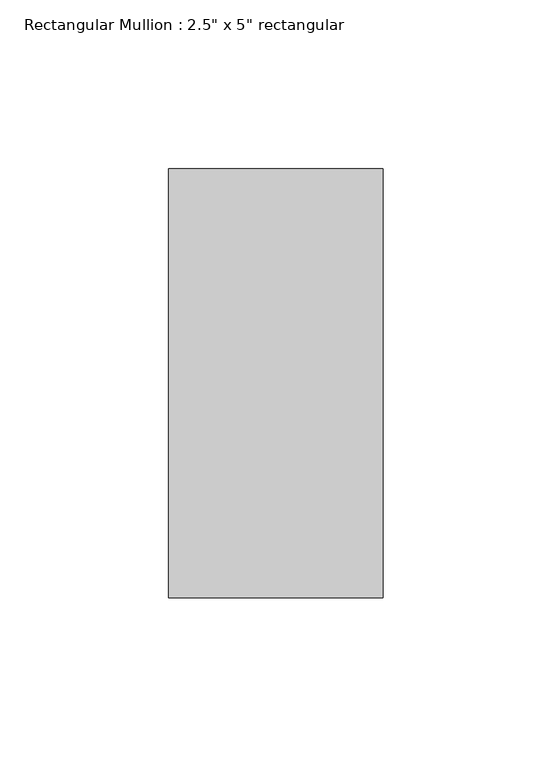
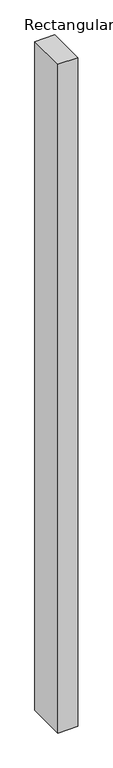
"""IFC4 building model written with IfcOpenShell, lengths in millimetres: member geometry."""

from ifc_helpers import new_model, si_unit, frame, origin, place, context, project, spatial, polyline, outline, extrude, source, transform, mapped, element, save


def member_3974447c(model_context):
    return source(origin(), model_context, "Body", "SweptSolid", [
        extrude(outline(polyline([(31.75, 63.5), (31.75, -63.5), (-31.75, -63.5), (-31.75, 63.5), (31.75, 63.5)])), frame((0.0, 0.0, -2254.3645985), z_axis=(0.0, 0.0, 1.0), x_axis=(1.0, 0.0, 0.0)), (0.0, 0.0, 1.0), 2254.3645985),
    ])


if __name__ == "__main__":
    model = new_model("IFC4")
    model_context = context("Model", 3, world=origin())
    ifc_project = project(units=[si_unit("LENGTHUNIT", "METRE", prefix="MILLI")], contexts=[model_context])
    site = spatial("IfcSite", under=ifc_project)
    building = spatial("IfcBuilding", under=site)
    placement = place(None, origin())
    member_shape = member_3974447c(model_context)
    element("IfcMember", 1, ObjectType="Rectangular Mullion : 2.5\" x 5\" rectangular", at=placement, inside=building, context=model_context, shape_type="MappedRepresentation", body=[
        mapped(member_shape, transform((0.0, 0.0, 0.0), x_axis=(1.0, 0.0, 0.0), y_axis=(0.0, 1.0, 0.0), z_axis=(0.0, 0.0, 1.0))),
    ])
    save(model, "model.ifc")

# Revit data of these elements
# Type "Rectangular Mullion : 2.5\" x 5\" rectangular"
#   built-in parameter 1007304 = 0.416667 (stored number, unit not read)
#   built-in parameter 1007301 = 0.104167 (stored number, unit not read)
#   built-in parameter 1007300 = 0.104167 (stored number, unit not read)
# Element 1 (IfcMember, "Rectangular Mullion : 2.5\" x 5\" rectangular")
#   Materials on its faces: "Aluminum"
# Materials
#   "Aluminum": class "Metal", colour RGB 247 247 247, transparency 0, Description = "Aluminum 6061", Cost = 0
